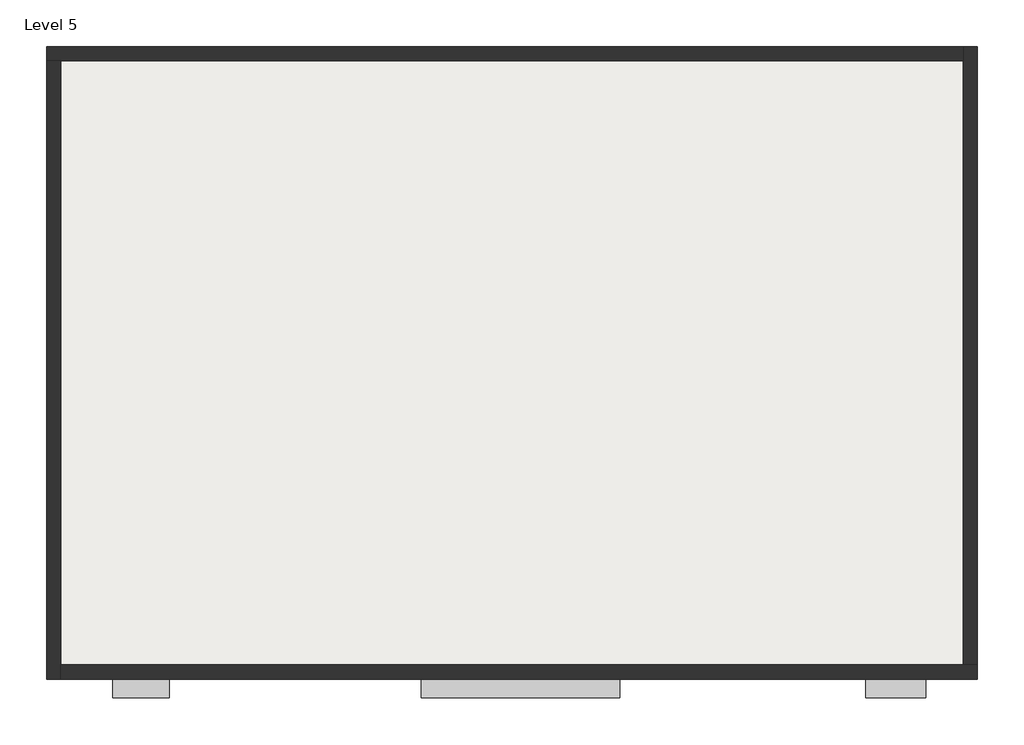
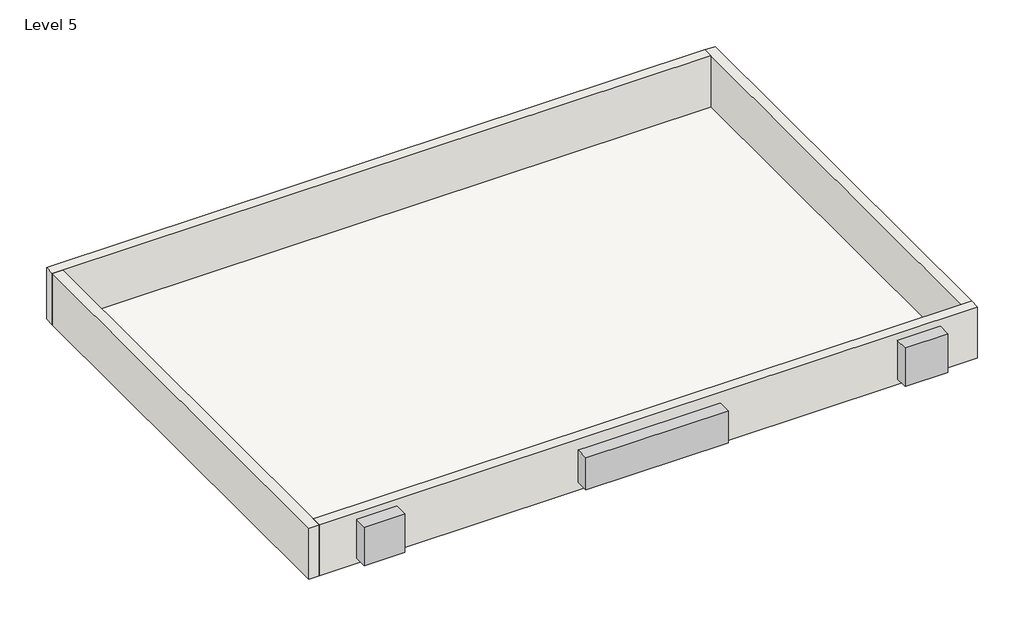
# One storey, incomplete: 4 walls, 1 proxy, 1 roof.
"""IFC4 building model written with IfcOpenShell, lengths in millimetres."""

from ifc_helpers import new_model, si_unit, frame, origin, place, context, project, spatial, polyline, outline, extrude, faceted_brep, transform, mapped, element, save
from components import generic_models_1_generic_models_1_6252d277

model = new_model("IFC4")

# Units and contexts
model_context = context("Model", 3, world=origin())
ifc_project = project(units=[si_unit("LENGTHUNIT", "METRE", prefix="MILLI")], contexts=[model_context])

# Site, building, storey
site = spatial("IfcSite", under=ifc_project)
building = spatial("IfcBuilding", under=site)
storey = spatial("IfcBuildingStorey", under=building, Name="Level 5", Elevation=9601.2)

# Proxy
placement = place(None, origin())
generic_models_1_generic_models_1_shape = generic_models_1_generic_models_1_6252d277(model_context)
element("IfcBuildingElementProxy", 1, Name="Generic Models 1 : Generic Models 1", ObjectType="Generic Models 1 : Generic Models 1", at=placement, inside=storey, context=model_context, shape_type="MappedRepresentation", body=[
    mapped(generic_models_1_generic_models_1_shape, transform((0.0, 0.0, 0.0), x_axis=(1.0, 0.0, 0.0), y_axis=(0.0, 1.0, 0.0), z_axis=(0.0, 0.0, 1.0))),
])

# Roof
element("IfcRoof", 2, ObjectType="Generic - 12\"", at=placement, inside=storey, context=model_context, shape_type="SweptSolid", body=[
    extrude(outline(polyline([(-7944.5640964, 7068.003532), (6625.5109036, 7068.003532), (6625.5109036, -2685.596468), (-7944.5640964, -2685.596468), (-7944.5640964, 7068.003532)])), frame((0.0, 0.0, 9448.8), z_axis=(0.0, 0.0, 1.0), x_axis=(1.0, 0.0, 0.0)), (0.0, 0.0, 1.0), 152.4),
])

# Walls
element("IfcWall", 3, ObjectType="WALL9\"", at=placement, inside=storey, context=model_context, shape_type="Brep", body=[
    faceted_brep([(-8173.1640964, 7068.003532, 9601.2), (-7944.5640964, 7068.003532, 9601.2), (6625.5109036, 7068.003532, 9601.2), (6625.5109036, 7068.003532, 10820.4), (-7944.5640964, 7068.003532, 10820.4), (-8173.1640964, 7068.003532, 10820.4), (-8173.1640964, 7296.603532, 9601.2), (-8173.1640964, 7296.603532, 10820.4), (6625.5109036, 7296.603532, 10820.4), (6625.5109036, 7296.603532, 9601.2)], [[[0, 1, 2, 3, 4, 5]], [[6, 7, 8, 9]], [[2, 1, 0, 6, 9]], [[5, 4, 3, 8, 7]], [[0, 5, 7, 6]], [[3, 2, 9, 8]]]),
])
element("IfcWall", 4, ObjectType="WALL9\"", at=placement, inside=storey, context=model_context, shape_type="Brep", body=[
    faceted_brep([(-7944.5640964, -2914.196468, 9601.2), (-7944.5640964, -2685.596468, 9601.2), (-7944.5640964, 7068.003532, 9601.2), (-7944.5640964, 7068.003532, 10820.4), (-7944.5640964, -2685.596468, 10820.4), (-7944.5640964, -2914.196468, 10820.4), (-8173.1640964, -2914.196468, 9601.2), (-8173.1640964, -2914.196468, 10820.4), (-8173.1640964, 7068.003532, 10820.4), (-8173.1640964, 7068.003532, 9601.2)], [[[0, 1, 2, 3, 4, 5]], [[6, 7, 8, 9]], [[2, 1, 0, 6, 9]], [[5, 4, 3, 8, 7]], [[0, 5, 7, 6]], [[3, 2, 9, 8]]]),
])
element("IfcWall", 5, ObjectType="WALL9\"", at=placement, inside=storey, context=model_context, shape_type="Brep", body=[
    faceted_brep([(6854.1109036, -2685.596468, 9601.2), (6625.5109036, -2685.596468, 9601.2), (-7944.5640964, -2685.596468, 9601.2), (-7944.5640964, -2685.596468, 10820.4), (6625.5109036, -2685.596468, 10820.4), (6854.1109036, -2685.596468, 10820.4), (6854.1109036, -2914.196468, 9601.2), (6854.1109036, -2914.196468, 10820.4), (-7944.5640964, -2914.196468, 10820.4), (-7944.5640964, -2914.196468, 9601.2)], [[[0, 1, 2, 3, 4, 5]], [[6, 7, 8, 9]], [[2, 1, 0, 6, 9]], [[5, 4, 3, 8, 7]], [[0, 5, 7, 6]], [[3, 2, 9, 8]]]),
])
element("IfcWall", 6, ObjectType="WALL9\"", at=placement, inside=storey, context=model_context, shape_type="Brep", body=[
    faceted_brep([(6625.5109036, 7296.603532, 9601.2), (6625.5109036, 7068.003532, 9601.2), (6625.5109036, -2685.596468, 9601.2), (6625.5109036, -2685.596468, 10820.4), (6625.5109036, 7068.003532, 10820.4), (6625.5109036, 7296.603532, 10820.4), (6854.1109036, 7296.603532, 9601.2), (6854.1109036, 7296.603532, 10820.4), (6854.1109036, -2685.596468, 10820.4), (6854.1109036, -2685.596468, 9601.2)], [[[0, 1, 2, 3, 4, 5]], [[6, 7, 8, 9]], [[2, 1, 0, 6, 9]], [[5, 4, 3, 8, 7]], [[0, 5, 7, 6]], [[3, 2, 9, 8]]]),
])

save(model, "model.ifc")

# Revit data of these elements
# Type "Generic - 12\""
#   Assembly Code = "B1020"
#   Layers, outside or top first: 0' - 6" no material (function 1)
# Type "WALL9\""
#   Assembly Code = "B2010"
#   Layers, outside or top first: 0' - 9" no material (function 1)
# Element 1 (IfcBuildingElementProxy, "Generic Models 1 : Generic Models 1")
#   Phase Created = New Construction
#   Materials on its faces: "Parking Stripe", "Carpet (1)"
# Element 2 (IfcRoof, "Generic - 12\"")
#   built-in parameter 1001705 = 31.5 (stored number, unit not read)
#   built-in parameter 1001701 = -0.5 (stored number, unit not read)
#   built-in parameter 1001710 = 33615
#   Phase Created = New Construction
#   Materials on its faces: "Default Roof"
# Elements 3, 4, 5, 6 (IfcWall, "WALL9\"")
#   Top Offset = 0' - 0"
#   Base Offset = 0' - 0"
#   Unconnected Height = 4' - 0"
#   wall height = 4' - 0"
#   Phase Created = New Construction
#   Base Constraint = Level 5
#   Materials on its faces: "Default Wall"
# Materials
#   "Parking Stripe": class "Paint", colour RGB 250 250 91, transparency 0, Cost = 0
#   "Carpet (1)": class "Carpet", colour RGB 124 80 67, transparency 0, Description = "Interior finish", Cost = 0
#   "Default Roof": colour RGB 88 101 114, transparency 0, Cost = 0
#   "Default Wall": colour RGB 128 128 128, transparency 0, Cost = 0
